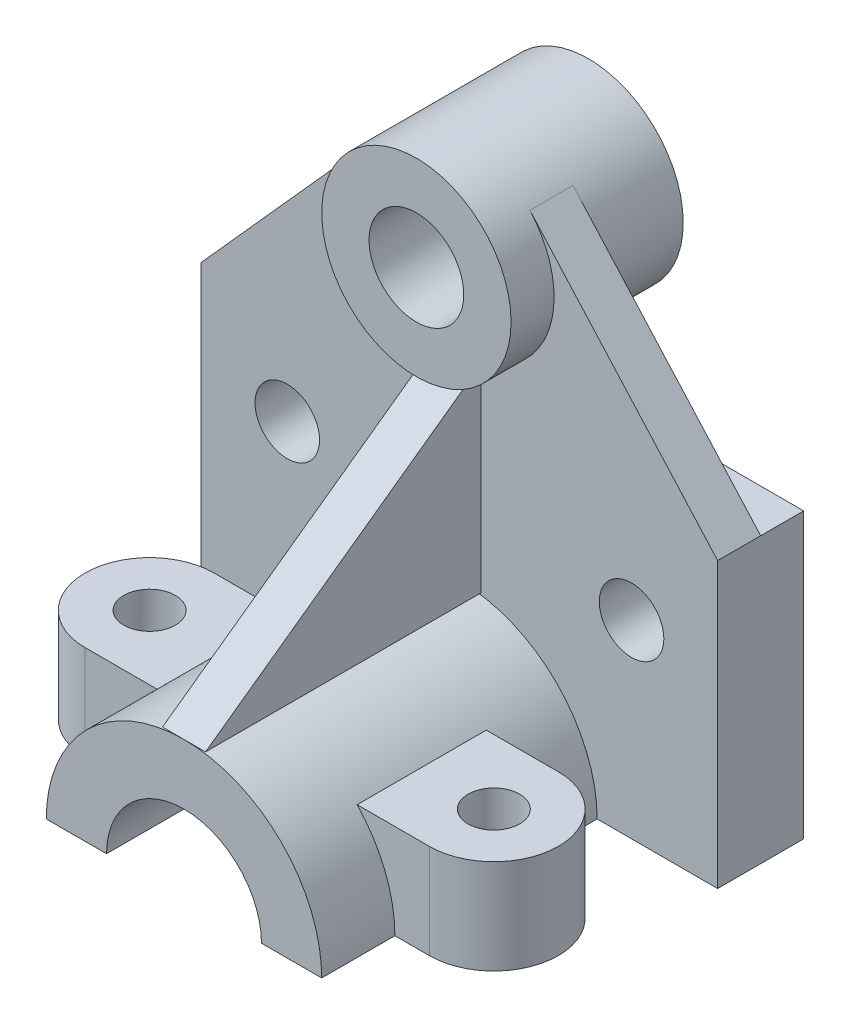
ISO-10303-21;
HEADER;
FILE_DESCRIPTION(('STEP AP214'),'2;1');
FILE_NAME('part.step','',(''),(''),'','','');
FILE_SCHEMA(('AUTOMOTIVE_DESIGN { 1 0 10303 214 1 1 1 1 }'));
ENDSEC;
DATA;
#1=APPLICATION_CONTEXT('core data for automotive mechanical design processes');
#2=APPLICATION_PROTOCOL_DEFINITION('international standard','automotive_design',2000,#1);
#3=PRODUCT_CONTEXT('',#1,'mechanical');
#4=PRODUCT('Part','Part','',(#3));
#5=PRODUCT_RELATED_PRODUCT_CATEGORY('part','',(#4));
#6=PRODUCT_DEFINITION_FORMATION('','',#4);
#7=PRODUCT_DEFINITION_CONTEXT('part definition',#1,'design');
#8=PRODUCT_DEFINITION('design','',#6,#7);
#9=PRODUCT_DEFINITION_SHAPE('','',#8);
#10=(LENGTH_UNIT() NAMED_UNIT(*) SI_UNIT(.MILLI.,.METRE.));
#11=(NAMED_UNIT(*) PLANE_ANGLE_UNIT() SI_UNIT($,.RADIAN.));
#12=(NAMED_UNIT(*) SI_UNIT($,.STERADIAN.) SOLID_ANGLE_UNIT());
#13=UNCERTAINTY_MEASURE_WITH_UNIT(LENGTH_MEASURE(1.E-05),#10,'distance_accuracy_value','');
#14=(GEOMETRIC_REPRESENTATION_CONTEXT(3) GLOBAL_UNCERTAINTY_ASSIGNED_CONTEXT((#13)) GLOBAL_UNIT_ASSIGNED_CONTEXT((#10,
#11,#12)) REPRESENTATION_CONTEXT('',''));
#15=CARTESIAN_POINT('',(0.,0.,0.));
#16=DIRECTION('',(0.,0.,1.));
#17=DIRECTION('',(1.,0.,0.));
#18=AXIS2_PLACEMENT_3D('',#15,#16,#17);
#19=CARTESIAN_POINT('',(120.,32.,0.));
#20=DIRECTION('',(0.,0.,-1.));
#21=DIRECTION('',(-1.,0.,0.));
#22=AXIS2_PLACEMENT_3D('',#19,#20,#21);
#23=PLANE('',#22);
#24=DIRECTION('',(0.,1.,0.));
#25=VECTOR('',#24,1.);
#26=CARTESIAN_POINT('',(65.,32.,0.));
#27=LINE('',#26,#25);
#28=CARTESIAN_POINT('',(65.,32.,0.));
#29=VERTEX_POINT('',#28);
#30=CARTESIAN_POINT('',(65.,78.,0.));
#31=VERTEX_POINT('',#30);
#32=EDGE_CURVE('E89',#29,#31,#27,.T.);
#33=ORIENTED_EDGE('',*,*,#32,.F.);
#34=DIRECTION('',(-1.,0.,0.));
#35=VECTOR('',#34,1.);
#36=CARTESIAN_POINT('',(120.,32.,0.));
#37=LINE('',#36,#35);
#38=CARTESIAN_POINT('',(55.,32.,0.));
#39=VERTEX_POINT('',#38);
#40=EDGE_CURVE('E58',#29,#39,#37,.T.);
#41=ORIENTED_EDGE('',*,*,#40,.T.);
#42=DIRECTION('',(0.,-1.,0.));
#43=VECTOR('',#42,1.);
#44=CARTESIAN_POINT('',(55.,32.,0.));
#45=LINE('',#44,#43);
#46=CARTESIAN_POINT('',(55.,78.,0.));
#47=VERTEX_POINT('',#46);
#48=EDGE_CURVE('E101',#47,#39,#45,.T.);
#49=ORIENTED_EDGE('',*,*,#48,.F.);
#50=DIRECTION('',(-1.,0.,0.));
#51=VECTOR('',#50,1.);
#52=CARTESIAN_POINT('',(120.,78.,0.));
#53=LINE('',#52,#51);
#54=EDGE_CURVE('E12',#31,#47,#53,.T.);
#55=ORIENTED_EDGE('',*,*,#54,.F.);
#56=EDGE_LOOP('',(#33,#41,#49,#55));
#57=FACE_BOUND('',#56,.T.);
#58=ADVANCED_FACE('F60',(#57),#23,.T.);
#59=CARTESIAN_POINT('',(120.,78.,0.));
#60=DIRECTION('',(0.,0.812015371342713,0.583636048152576));
#61=DIRECTION('',(0.,-0.583636048152576,0.812015371342713));
#62=AXIS2_PLACEMENT_3D('',#59,#60,#61);
#63=PLANE('',#62);
#64=DIRECTION('',(0.,-0.583636048152575,0.812015371342713));
#65=VECTOR('',#64,1.);
#66=CARTESIAN_POINT('',(65.,78.,0.));
#67=LINE('',#66,#65);
#68=CARTESIAN_POINT('',(65.,32.,64.));
#69=VERTEX_POINT('',#68);
#70=EDGE_CURVE('E71',#31,#69,#67,.T.);
#71=ORIENTED_EDGE('',*,*,#70,.F.);
#72=ORIENTED_EDGE('',*,*,#54,.T.);
#73=DIRECTION('',(0.,0.583636048152575,-0.812015371342713));
#74=VECTOR('',#73,1.);
#75=CARTESIAN_POINT('',(55.,78.,0.));
#76=LINE('',#75,#74);
#77=CARTESIAN_POINT('',(55.,32.,64.));
#78=VERTEX_POINT('',#77);
#79=EDGE_CURVE('E110',#78,#47,#76,.T.);
#80=ORIENTED_EDGE('',*,*,#79,.F.);
#81=DIRECTION('',(-1.,0.,0.));
#82=VECTOR('',#81,1.);
#83=CARTESIAN_POINT('',(120.,32.,64.));
#84=LINE('',#83,#82);
#85=EDGE_CURVE('E61',#69,#78,#84,.T.);
#86=ORIENTED_EDGE('',*,*,#85,.F.);
#87=EDGE_LOOP('',(#71,#72,#80,#86));
#88=FACE_BOUND('',#87,.T.);
#89=ADVANCED_FACE('F100',(#88),#63,.T.);
#90=CARTESIAN_POINT('',(120.,32.,64.));
#91=DIRECTION('',(0.,-1.,0.));
#92=DIRECTION('',(0.,0.,-1.));
#93=AXIS2_PLACEMENT_3D('',#90,#91,#92);
#94=PLANE('',#93);
#95=DIRECTION('',(0.,0.,-1.));
#96=VECTOR('',#95,1.);
#97=CARTESIAN_POINT('',(65.,32.,64.));
#98=LINE('',#97,#96);
#99=EDGE_CURVE('E95',#69,#29,#98,.T.);
#100=ORIENTED_EDGE('',*,*,#99,.F.);
#101=ORIENTED_EDGE('',*,*,#85,.T.);
#102=DIRECTION('',(0.,0.,1.));
#103=VECTOR('',#102,1.);
#104=CARTESIAN_POINT('',(55.,32.,64.));
#105=LINE('',#104,#103);
#106=EDGE_CURVE('E104',#39,#78,#105,.T.);
#107=ORIENTED_EDGE('',*,*,#106,.F.);
#108=ORIENTED_EDGE('',*,*,#40,.F.);
#109=EDGE_LOOP('',(#100,#101,#107,#108));
#110=FACE_BOUND('',#109,.T.);
#111=ADVANCED_FACE('F115',(#110),#94,.T.);
#112=CARTESIAN_POINT('',(55.,0.,0.));
#113=DIRECTION('',(-1.,0.,0.));
#114=DIRECTION('',(0.,0.,1.));
#115=AXIS2_PLACEMENT_3D('',#112,#113,#114);
#116=PLANE('',#115);
#117=ORIENTED_EDGE('',*,*,#48,.T.);
#118=ORIENTED_EDGE('',*,*,#106,.T.);
#119=ORIENTED_EDGE('',*,*,#79,.T.);
#120=EDGE_LOOP('',(#117,#118,#119));
#121=FACE_BOUND('',#120,.T.);
#122=ADVANCED_FACE('F114',(#121),#116,.T.);
#123=CARTESIAN_POINT('',(65.,0.,0.));
#124=DIRECTION('',(-1.,0.,0.));
#125=DIRECTION('',(0.,0.,1.));
#126=AXIS2_PLACEMENT_3D('',#123,#124,#125);
#127=PLANE('',#126);
#128=ORIENTED_EDGE('',*,*,#32,.T.);
#129=ORIENTED_EDGE('',*,*,#70,.T.);
#130=ORIENTED_EDGE('',*,*,#99,.T.);
#131=EDGE_LOOP('',(#128,#129,#130));
#132=FACE_BOUND('',#131,.T.);
#133=ADVANCED_FACE('F93',(#132),#127,.F.);
#134=CLOSED_SHELL('',(#58,#89,#111,#122,#133));
#135=MANIFOLD_SOLID_BREP('B2',#134);
#136=CARTESIAN_POINT('',(60.,0.,64.));
#137=DIRECTION('',(0.,0.,-1.));
#138=DIRECTION('',(-1.,0.,0.));
#139=AXIS2_PLACEMENT_3D('',#136,#137,#138);
#140=CYLINDRICAL_SURFACE('',#139,32.);
#141=CARTESIAN_POINT('',(60.,0.,17.));
#142=DIRECTION('',(0.,0.,1.));
#143=DIRECTION('',(1.,0.,0.));
#144=AXIS2_PLACEMENT_3D('',#141,#142,#143);
#145=CIRCLE('',#144,32.);
#146=CARTESIAN_POINT('',(36.7620999227555,22.,17.));
#147=VERTEX_POINT('',#146);
#148=CARTESIAN_POINT('',(28.,0.,17.));
#149=VERTEX_POINT('',#148);
#150=EDGE_CURVE('E318',#147,#149,#145,.T.);
#151=ORIENTED_EDGE('',*,*,#150,.F.);
#152=DIRECTION('',(0.,0.,-1.));
#153=VECTOR('',#152,1.);
#154=CARTESIAN_POINT('',(36.7620999227555,22.,64.));
#155=LINE('',#154,#153);
#156=CARTESIAN_POINT('',(36.7620999227555,22.,47.));
#157=VERTEX_POINT('',#156);
#158=EDGE_CURVE('E54',#157,#147,#155,.T.);
#159=ORIENTED_EDGE('',*,*,#158,.F.);
#160=CARTESIAN_POINT('',(60.,0.,47.));
#161=DIRECTION('',(0.,0.,-1.));
#162=DIRECTION('',(-1.,0.,0.));
#163=AXIS2_PLACEMENT_3D('',#160,#161,#162);
#164=CIRCLE('',#163,32.);
#165=CARTESIAN_POINT('',(28.,0.,47.));
#166=VERTEX_POINT('',#165);
#167=EDGE_CURVE('E296',#166,#157,#164,.T.);
#168=ORIENTED_EDGE('',*,*,#167,.F.);
#169=DIRECTION('',(0.,0.,-1.));
#170=VECTOR('',#169,1.);
#171=CARTESIAN_POINT('',(28.,0.,64.));
#172=LINE('',#171,#170);
#173=CARTESIAN_POINT('',(28.,0.,64.));
#174=VERTEX_POINT('',#173);
#175=EDGE_CURVE('E409',#174,#166,#172,.T.);
#176=ORIENTED_EDGE('',*,*,#175,.F.);
#177=CARTESIAN_POINT('',(60.,0.,64.));
#178=DIRECTION('',(0.,0.,1.));
#179=DIRECTION('',(1.,0.,0.));
#180=AXIS2_PLACEMENT_3D('',#177,#178,#179);
#181=CIRCLE('',#180,32.);
#182=CARTESIAN_POINT('',(92.,0.,64.));
#183=VERTEX_POINT('',#182);
#184=EDGE_CURVE('E396',#183,#174,#181,.T.);
#185=ORIENTED_EDGE('',*,*,#184,.F.);
#186=DIRECTION('',(0.,0.,-1.));
#187=VECTOR('',#186,1.);
#188=CARTESIAN_POINT('',(92.,0.,64.));
#189=LINE('',#188,#187);
#190=CARTESIAN_POINT('',(92.,0.,47.));
#191=VERTEX_POINT('',#190);
#192=EDGE_CURVE('E407',#183,#191,#189,.T.);
#193=ORIENTED_EDGE('',*,*,#192,.T.);
#194=CARTESIAN_POINT('',(60.,0.,47.));
#195=DIRECTION('',(0.,0.,1.));
#196=DIRECTION('',(1.,0.,0.));
#197=AXIS2_PLACEMENT_3D('',#194,#195,#196);
#198=CIRCLE('',#197,32.);
#199=CARTESIAN_POINT('',(83.2379000772445,22.,47.));
#200=VERTEX_POINT('',#199);
#201=EDGE_CURVE('E178',#191,#200,#198,.T.);
#202=ORIENTED_EDGE('',*,*,#201,.T.);
#203=DIRECTION('',(0.,0.,-1.));
#204=VECTOR('',#203,1.);
#205=CARTESIAN_POINT('',(83.2379000772445,22.,64.));
#206=LINE('',#205,#204);
#207=CARTESIAN_POINT('',(83.2379000772445,22.,17.));
#208=VERTEX_POINT('',#207);
#209=EDGE_CURVE('E162',#208,#200,#206,.F.);
#210=ORIENTED_EDGE('',*,*,#209,.F.);
#211=CARTESIAN_POINT('',(60.,0.,17.));
#212=DIRECTION('',(0.,0.,-1.));
#213=DIRECTION('',(-1.,0.,0.));
#214=AXIS2_PLACEMENT_3D('',#211,#212,#213);
#215=CIRCLE('',#214,32.);
#216=CARTESIAN_POINT('',(92.,0.,17.));
#217=VERTEX_POINT('',#216);
#218=EDGE_CURVE('E345',#208,#217,#215,.T.);
#219=ORIENTED_EDGE('',*,*,#218,.T.);
#220=CARTESIAN_POINT('',(92.,0.,0.));
#221=VERTEX_POINT('',#220);
#222=EDGE_CURVE('E401',#217,#221,#189,.T.);
#223=ORIENTED_EDGE('',*,*,#222,.T.);
#224=CARTESIAN_POINT('',(60.,0.,0.));
#225=DIRECTION('',(0.,0.,1.));
#226=DIRECTION('',(1.,0.,0.));
#227=AXIS2_PLACEMENT_3D('',#224,#225,#226);
#228=CIRCLE('',#227,32.);
#229=CARTESIAN_POINT('',(28.,0.,0.));
#230=VERTEX_POINT('',#229);
#231=EDGE_CURVE('E394',#221,#230,#228,.T.);
#232=ORIENTED_EDGE('',*,*,#231,.T.);
#233=EDGE_CURVE('E408',#149,#230,#172,.T.);
#234=ORIENTED_EDGE('',*,*,#233,.F.);
#235=EDGE_LOOP('',(#151,#159,#168,#176,#185,#193,#202,#210,#219,#223,#232,#234));
#236=FACE_BOUND('',#235,.T.);
#237=ADVANCED_FACE('F154',(#236),#140,.T.);
#238=CARTESIAN_POINT('',(0.,66.,-20.));
#239=DIRECTION('',(-1.,0.,0.));
#240=DIRECTION('',(0.,0.,1.));
#241=AXIS2_PLACEMENT_3D('',#238,#239,#240);
#242=PLANE('',#241);
#243=DIRECTION('',(0.,-1.,0.));
#244=VECTOR('',#243,1.);
#245=CARTESIAN_POINT('',(0.,66.,0.));
#246=LINE('',#245,#244);
#247=CARTESIAN_POINT('',(0.,66.,0.));
#248=VERTEX_POINT('',#247);
#249=CARTESIAN_POINT('',(0.,0.,0.));
#250=VERTEX_POINT('',#249);
#251=EDGE_CURVE('E415',#248,#250,#246,.T.);
#252=ORIENTED_EDGE('',*,*,#251,.F.);
#253=DIRECTION('',(0.,0.,1.));
#254=VECTOR('',#253,1.);
#255=CARTESIAN_POINT('',(0.,66.,-10.));
#256=LINE('',#255,#254);
#257=CARTESIAN_POINT('',(0.,66.,-10.));
#258=VERTEX_POINT('',#257);
#259=EDGE_CURVE('E378',#258,#248,#256,.T.);
#260=ORIENTED_EDGE('',*,*,#259,.F.);
#261=DIRECTION('',(0.,0.,1.));
#262=VECTOR('',#261,1.);
#263=CARTESIAN_POINT('',(0.,66.,-20.));
#264=LINE('',#263,#262);
#265=CARTESIAN_POINT('',(0.,66.,-20.));
#266=VERTEX_POINT('',#265);
#267=EDGE_CURVE('E434',#266,#258,#264,.T.);
#268=ORIENTED_EDGE('',*,*,#267,.F.);
#269=DIRECTION('',(0.,-1.,0.));
#270=VECTOR('',#269,1.);
#271=CARTESIAN_POINT('',(0.,66.,-20.));
#272=LINE('',#271,#270);
#273=CARTESIAN_POINT('',(0.,0.,-20.));
#274=VERTEX_POINT('',#273);
#275=EDGE_CURVE('E413',#266,#274,#272,.T.);
#276=ORIENTED_EDGE('',*,*,#275,.T.);
#277=DIRECTION('',(0.,0.,1.));
#278=VECTOR('',#277,1.);
#279=CARTESIAN_POINT('',(0.,0.,-20.));
#280=LINE('',#279,#278);
#281=EDGE_CURVE('E426',#274,#250,#280,.T.);
#282=ORIENTED_EDGE('',*,*,#281,.T.);
#283=EDGE_LOOP('',(#252,#260,#268,#276,#282));
#284=FACE_BOUND('',#283,.T.);
#285=ADVANCED_FACE('F160',(#284),#242,.T.);
#286=CARTESIAN_POINT('',(120.,66.,-20.));
#287=DIRECTION('',(0.,1.,0.));
#288=DIRECTION('',(0.,0.,1.));
#289=AXIS2_PLACEMENT_3D('',#286,#287,#288);
#290=PLANE('',#289);
#291=DIRECTION('',(-1.,0.,0.));
#292=VECTOR('',#291,1.);
#293=CARTESIAN_POINT('',(0.,66.,-10.));
#294=LINE('',#293,#292);
#295=CARTESIAN_POINT('',(120.,66.,-10.));
#296=VERTEX_POINT('',#295);
#297=EDGE_CURVE('E362',#296,#258,#294,.T.);
#298=ORIENTED_EDGE('',*,*,#297,.F.);
#299=DIRECTION('',(0.,0.,1.));
#300=VECTOR('',#299,1.);
#301=CARTESIAN_POINT('',(120.,66.,-20.));
#302=LINE('',#301,#300);
#303=CARTESIAN_POINT('',(120.,66.,-20.));
#304=VERTEX_POINT('',#303);
#305=EDGE_CURVE('E437',#304,#296,#302,.T.);
#306=ORIENTED_EDGE('',*,*,#305,.F.);
#307=DIRECTION('',(-1.,0.,0.));
#308=VECTOR('',#307,1.);
#309=CARTESIAN_POINT('',(120.,66.,-20.));
#310=LINE('',#309,#308);
#311=EDGE_CURVE('E421',#304,#266,#310,.T.);
#312=ORIENTED_EDGE('',*,*,#311,.T.);
#313=ORIENTED_EDGE('',*,*,#267,.T.);
#314=EDGE_LOOP('',(#298,#306,#312,#313));
#315=FACE_BOUND('',#314,.T.);
#316=ADVANCED_FACE('F500',(#315),#290,.T.);
#317=CARTESIAN_POINT('',(120.,0.,-20.));
#318=DIRECTION('',(1.,0.,0.));
#319=DIRECTION('',(0.,0.,-1.));
#320=AXIS2_PLACEMENT_3D('',#317,#318,#319);
#321=PLANE('',#320);
#322=DIRECTION('',(0.,1.,0.));
#323=VECTOR('',#322,1.);
#324=CARTESIAN_POINT('',(120.,0.,0.));
#325=LINE('',#324,#323);
#326=CARTESIAN_POINT('',(120.,0.,0.));
#327=VERTEX_POINT('',#326);
#328=CARTESIAN_POINT('',(120.,66.,0.));
#329=VERTEX_POINT('',#328);
#330=EDGE_CURVE('E417',#327,#329,#325,.T.);
#331=ORIENTED_EDGE('',*,*,#330,.F.);
#332=DIRECTION('',(0.,0.,1.));
#333=VECTOR('',#332,1.);
#334=CARTESIAN_POINT('',(120.,0.,-20.));
#335=LINE('',#334,#333);
#336=CARTESIAN_POINT('',(120.,0.,-20.));
#337=VERTEX_POINT('',#336);
#338=EDGE_CURVE('E442',#337,#327,#335,.T.);
#339=ORIENTED_EDGE('',*,*,#338,.F.);
#340=DIRECTION('',(0.,1.,0.));
#341=VECTOR('',#340,1.);
#342=CARTESIAN_POINT('',(120.,0.,-20.));
#343=LINE('',#342,#341);
#344=EDGE_CURVE('E419',#337,#304,#343,.T.);
#345=ORIENTED_EDGE('',*,*,#344,.T.);
#346=ORIENTED_EDGE('',*,*,#305,.T.);
#347=DIRECTION('',(0.,0.,1.));
#348=VECTOR('',#347,1.);
#349=CARTESIAN_POINT('',(120.,66.,-10.));
#350=LINE('',#349,#348);
#351=EDGE_CURVE('E376',#296,#329,#350,.T.);
#352=ORIENTED_EDGE('',*,*,#351,.T.);
#353=EDGE_LOOP('',(#331,#339,#345,#346,#352));
#354=FACE_BOUND('',#353,.T.);
#355=ADVANCED_FACE('F478',(#354),#321,.T.);
#356=CARTESIAN_POINT('',(0.,0.,-20.));
#357=DIRECTION('',(0.,-1.,0.));
#358=DIRECTION('',(0.,0.,-1.));
#359=AXIS2_PLACEMENT_3D('',#356,#357,#358);
#360=PLANE('',#359);
#361=CARTESIAN_POINT('',(20.,0.,32.));
#362=DIRECTION('',(0.,-1.,0.));
#363=DIRECTION('',(0.,0.,-1.));
#364=AXIS2_PLACEMENT_3D('',#361,#362,#363);
#365=CIRCLE('',#364,6.);
#366=CARTESIAN_POINT('',(20.,0.,26.));
#367=VERTEX_POINT('',#366);
#368=EDGE_CURVE('E518',#367,#367,#365,.T.);
#369=ORIENTED_EDGE('',*,*,#368,.F.);
#370=EDGE_LOOP('',(#369));
#371=FACE_BOUND('',#370,.T.);
#372=CARTESIAN_POINT('',(100.,0.,32.));
#373=DIRECTION('',(0.,-1.,0.));
#374=DIRECTION('',(0.,0.,-1.));
#375=AXIS2_PLACEMENT_3D('',#372,#373,#374);
#376=CIRCLE('',#375,6.);
#377=CARTESIAN_POINT('',(100.,0.,26.));
#378=VERTEX_POINT('',#377);
#379=EDGE_CURVE('E511',#378,#378,#376,.T.);
#380=ORIENTED_EDGE('',*,*,#379,.F.);
#381=EDGE_LOOP('',(#380));
#382=FACE_BOUND('',#381,.T.);
#383=DIRECTION('',(-1.,0.,0.));
#384=VECTOR('',#383,1.);
#385=CARTESIAN_POINT('',(0.,0.,17.));
#386=LINE('',#385,#384);
#387=CARTESIAN_POINT('',(20.,0.,17.));
#388=VERTEX_POINT('',#387);
#389=EDGE_CURVE('E168',#149,#388,#386,.T.);
#390=ORIENTED_EDGE('',*,*,#389,.F.);
#391=ORIENTED_EDGE('',*,*,#233,.T.);
#392=DIRECTION('',(1.,0.,0.));
#393=VECTOR('',#392,1.);
#394=CARTESIAN_POINT('',(0.,0.,0.));
#395=LINE('',#394,#393);
#396=EDGE_CURVE('E429',#250,#230,#395,.T.);
#397=ORIENTED_EDGE('',*,*,#396,.F.);
#398=ORIENTED_EDGE('',*,*,#281,.F.);
#399=DIRECTION('',(1.,0.,0.));
#400=VECTOR('',#399,1.);
#401=CARTESIAN_POINT('',(0.,0.,-20.));
#402=LINE('',#401,#400);
#403=EDGE_CURVE('E418',#274,#337,#402,.T.);
#404=ORIENTED_EDGE('',*,*,#403,.T.);
#405=ORIENTED_EDGE('',*,*,#338,.T.);
#406=EDGE_CURVE('E427',#221,#327,#395,.T.);
#407=ORIENTED_EDGE('',*,*,#406,.F.);
#408=ORIENTED_EDGE('',*,*,#222,.F.);
#409=DIRECTION('',(1.,0.,0.));
#410=VECTOR('',#409,1.);
#411=CARTESIAN_POINT('',(0.,0.,17.));
#412=LINE('',#411,#410);
#413=CARTESIAN_POINT('',(100.,0.,17.));
#414=VERTEX_POINT('',#413);
#415=EDGE_CURVE('E319',#217,#414,#412,.T.);
#416=ORIENTED_EDGE('',*,*,#415,.T.);
#417=CARTESIAN_POINT('',(100.,0.,32.));
#418=DIRECTION('',(0.,-1.,0.));
#419=DIRECTION('',(0.,0.,-1.));
#420=AXIS2_PLACEMENT_3D('',#417,#418,#419);
#421=CIRCLE('',#420,15.);
#422=CARTESIAN_POINT('',(100.,0.,47.));
#423=VERTEX_POINT('',#422);
#424=EDGE_CURVE('E335',#414,#423,#421,.T.);
#425=ORIENTED_EDGE('',*,*,#424,.T.);
#426=DIRECTION('',(-1.,0.,0.));
#427=VECTOR('',#426,1.);
#428=CARTESIAN_POINT('',(0.,0.,47.));
#429=LINE('',#428,#427);
#430=EDGE_CURVE('E322',#423,#191,#429,.T.);
#431=ORIENTED_EDGE('',*,*,#430,.T.);
#432=ORIENTED_EDGE('',*,*,#192,.F.);
#433=DIRECTION('',(1.,0.,0.));
#434=VECTOR('',#433,1.);
#435=CARTESIAN_POINT('',(28.,0.,64.));
#436=LINE('',#435,#434);
#437=CARTESIAN_POINT('',(78.,0.,64.));
#438=VERTEX_POINT('',#437);
#439=EDGE_CURVE('E397',#438,#183,#436,.T.);
#440=ORIENTED_EDGE('',*,*,#439,.F.);
#441=DIRECTION('',(0.,0.,1.));
#442=VECTOR('',#441,1.);
#443=CARTESIAN_POINT('',(78.,0.,0.));
#444=LINE('',#443,#442);
#445=CARTESIAN_POINT('',(78.,0.,0.));
#446=VERTEX_POINT('',#445);
#447=EDGE_CURVE('E395',#446,#438,#444,.T.);
#448=ORIENTED_EDGE('',*,*,#447,.F.);
#449=DIRECTION('',(1.,0.,0.));
#450=VECTOR('',#449,1.);
#451=CARTESIAN_POINT('',(42.,0.,0.));
#452=LINE('',#451,#450);
#453=CARTESIAN_POINT('',(42.,0.,0.));
#454=VERTEX_POINT('',#453);
#455=EDGE_CURVE('E387',#454,#446,#452,.T.);
#456=ORIENTED_EDGE('',*,*,#455,.F.);
#457=DIRECTION('',(0.,0.,1.));
#458=VECTOR('',#457,1.);
#459=CARTESIAN_POINT('',(42.,0.,0.));
#460=LINE('',#459,#458);
#461=CARTESIAN_POINT('',(42.,0.,64.));
#462=VERTEX_POINT('',#461);
#463=EDGE_CURVE('E386',#454,#462,#460,.T.);
#464=ORIENTED_EDGE('',*,*,#463,.T.);
#465=EDGE_CURVE('E399',#174,#462,#436,.T.);
#466=ORIENTED_EDGE('',*,*,#465,.F.);
#467=ORIENTED_EDGE('',*,*,#175,.T.);
#468=DIRECTION('',(1.,0.,0.));
#469=VECTOR('',#468,1.);
#470=CARTESIAN_POINT('',(0.,0.,47.));
#471=LINE('',#470,#469);
#472=CARTESIAN_POINT('',(20.,0.,47.));
#473=VERTEX_POINT('',#472);
#474=EDGE_CURVE('E315',#473,#166,#471,.T.);
#475=ORIENTED_EDGE('',*,*,#474,.F.);
#476=CARTESIAN_POINT('',(20.,0.,32.));
#477=DIRECTION('',(0.,-1.,0.));
#478=DIRECTION('',(0.,0.,-1.));
#479=AXIS2_PLACEMENT_3D('',#476,#477,#478);
#480=CIRCLE('',#479,15.);
#481=EDGE_CURVE('E292',#473,#388,#480,.T.);
#482=ORIENTED_EDGE('',*,*,#481,.T.);
#483=EDGE_LOOP('',(#390,#391,#397,#398,#404,#405,#407,#408,#416,#425,#431,#432,#440,#448,#456,
#464,#466,#467,#475,#482));
#484=FACE_BOUND('',#483,.T.);
#485=ADVANCED_FACE('F473',(#371,#382,#484),#360,.T.);
#486=CARTESIAN_POINT('',(0.,0.,-20.));
#487=DIRECTION('',(0.,0.,1.));
#488=DIRECTION('',(1.,0.,0.));
#489=AXIS2_PLACEMENT_3D('',#486,#487,#488);
#490=PLANE('',#489);
#491=CARTESIAN_POINT('',(20.,44.,-20.));
#492=DIRECTION('',(0.,0.,1.));
#493=DIRECTION('',(1.,0.,0.));
#494=AXIS2_PLACEMENT_3D('',#491,#492,#493);
#495=CIRCLE('',#494,7.5);
#496=CARTESIAN_POINT('',(27.5,44.,-20.));
#497=VERTEX_POINT('',#496);
#498=EDGE_CURVE('E311',#497,#497,#495,.T.);
#499=ORIENTED_EDGE('',*,*,#498,.T.);
#500=EDGE_LOOP('',(#499));
#501=FACE_BOUND('',#500,.T.);
#502=CARTESIAN_POINT('',(100.,44.,-20.));
#503=DIRECTION('',(0.,0.,1.));
#504=DIRECTION('',(1.,0.,0.));
#505=AXIS2_PLACEMENT_3D('',#502,#503,#504);
#506=CIRCLE('',#505,7.5);
#507=CARTESIAN_POINT('',(107.5,44.,-20.));
#508=VERTEX_POINT('',#507);
#509=EDGE_CURVE('E506',#508,#508,#506,.T.);
#510=ORIENTED_EDGE('',*,*,#509,.T.);
#511=EDGE_LOOP('',(#510));
#512=FACE_BOUND('',#511,.T.);
#513=ORIENTED_EDGE('',*,*,#275,.F.);
#514=ORIENTED_EDGE('',*,*,#311,.F.);
#515=ORIENTED_EDGE('',*,*,#344,.F.);
#516=ORIENTED_EDGE('',*,*,#403,.F.);
#517=EDGE_LOOP('',(#513,#514,#515,#516));
#518=FACE_BOUND('',#517,.T.);
#519=ADVANCED_FACE('F498',(#501,#512,#518),#490,.F.);
#520=CARTESIAN_POINT('',(0.,0.,0.));
#521=DIRECTION('',(0.,0.,1.));
#522=DIRECTION('',(1.,0.,0.));
#523=AXIS2_PLACEMENT_3D('',#520,#521,#522);
#524=PLANE('',#523);
#525=CARTESIAN_POINT('',(20.,44.,0.));
#526=DIRECTION('',(0.,0.,1.));
#527=DIRECTION('',(1.,0.,0.));
#528=AXIS2_PLACEMENT_3D('',#525,#526,#527);
#529=CIRCLE('',#528,7.5);
#530=CARTESIAN_POINT('',(27.5,44.,0.));
#531=VERTEX_POINT('',#530);
#532=EDGE_CURVE('E507',#531,#531,#529,.T.);
#533=ORIENTED_EDGE('',*,*,#532,.F.);
#534=EDGE_LOOP('',(#533));
#535=FACE_BOUND('',#534,.T.);
#536=CARTESIAN_POINT('',(100.,44.,0.));
#537=DIRECTION('',(0.,0.,1.));
#538=DIRECTION('',(1.,0.,0.));
#539=AXIS2_PLACEMENT_3D('',#536,#537,#538);
#540=CIRCLE('',#539,7.5);
#541=CARTESIAN_POINT('',(107.5,44.,0.));
#542=VERTEX_POINT('',#541);
#543=EDGE_CURVE('E509',#542,#542,#540,.T.);
#544=ORIENTED_EDGE('',*,*,#543,.F.);
#545=EDGE_LOOP('',(#544));
#546=FACE_BOUND('',#545,.T.);
#547=DIRECTION('',(-0.667290225653567,0.744797794537021,0.));
#548=VECTOR('',#547,1.);
#549=CARTESIAN_POINT('',(99.368605602936,89.0277867926307,0.));
#550=LINE('',#549,#548);
#551=CARTESIAN_POINT('',(76.3855514798145,114.680384964378,0.));
#552=VERTEX_POINT('',#551);
#553=EDGE_CURVE('E361',#329,#552,#550,.T.);
#554=ORIENTED_EDGE('',*,*,#553,.T.);
#555=CARTESIAN_POINT('',(60.,100.,0.));
#556=DIRECTION('',(0.,0.,1.));
#557=DIRECTION('',(1.,0.,0.));
#558=AXIS2_PLACEMENT_3D('',#555,#556,#557);
#559=CIRCLE('',#558,22.);
#560=CARTESIAN_POINT('',(43.6144485201855,114.680384964378,0.));
#561=VERTEX_POINT('',#560);
#562=EDGE_CURVE('E355',#561,#552,#559,.T.);
#563=ORIENTED_EDGE('',*,*,#562,.F.);
#564=DIRECTION('',(0.667290225653567,0.744797794537022,0.));
#565=VECTOR('',#564,1.);
#566=CARTESIAN_POINT('',(-32.8017550332706,29.388232186684,0.));
#567=LINE('',#566,#565);
#568=EDGE_CURVE('E356',#248,#561,#567,.T.);
#569=ORIENTED_EDGE('',*,*,#568,.F.);
#570=ORIENTED_EDGE('',*,*,#251,.T.);
#571=ORIENTED_EDGE('',*,*,#396,.T.);
#572=ORIENTED_EDGE('',*,*,#231,.F.);
#573=ORIENTED_EDGE('',*,*,#406,.T.);
#574=ORIENTED_EDGE('',*,*,#330,.T.);
#575=EDGE_LOOP('',(#554,#563,#569,#570,#571,#572,#573,#574));
#576=FACE_BOUND('',#575,.T.);
#577=ADVANCED_FACE('F467',(#535,#546,#576),#524,.T.);
#578=CARTESIAN_POINT('',(60.,0.,64.));
#579=DIRECTION('',(0.,0.,1.));
#580=DIRECTION('',(1.,0.,0.));
#581=AXIS2_PLACEMENT_3D('',#578,#579,#580);
#582=PLANE('',#581);
#583=CARTESIAN_POINT('',(60.,0.,64.));
#584=DIRECTION('',(0.,0.,1.));
#585=DIRECTION('',(1.,0.,0.));
#586=AXIS2_PLACEMENT_3D('',#583,#584,#585);
#587=CIRCLE('',#586,18.);
#588=EDGE_CURVE('E374',#438,#462,#587,.T.);
#589=ORIENTED_EDGE('',*,*,#588,.F.);
#590=ORIENTED_EDGE('',*,*,#439,.T.);
#591=ORIENTED_EDGE('',*,*,#184,.T.);
#592=ORIENTED_EDGE('',*,*,#465,.T.);
#593=EDGE_LOOP('',(#589,#590,#591,#592));
#594=FACE_BOUND('',#593,.T.);
#595=ADVANCED_FACE('F548',(#594),#582,.T.);
#596=CARTESIAN_POINT('',(60.,0.,0.));
#597=DIRECTION('',(0.,0.,1.));
#598=DIRECTION('',(1.,0.,0.));
#599=AXIS2_PLACEMENT_3D('',#596,#597,#598);
#600=CYLINDRICAL_SURFACE('',#599,18.);
#601=ORIENTED_EDGE('',*,*,#588,.T.);
#602=ORIENTED_EDGE('',*,*,#463,.F.);
#603=CARTESIAN_POINT('',(60.,0.,0.));
#604=DIRECTION('',(0.,0.,1.));
#605=DIRECTION('',(1.,0.,0.));
#606=AXIS2_PLACEMENT_3D('',#603,#604,#605);
#607=CIRCLE('',#606,18.);
#608=EDGE_CURVE('E382',#446,#454,#607,.T.);
#609=ORIENTED_EDGE('',*,*,#608,.F.);
#610=ORIENTED_EDGE('',*,*,#447,.T.);
#611=EDGE_LOOP('',(#601,#602,#609,#610));
#612=FACE_BOUND('',#611,.T.);
#613=ADVANCED_FACE('F604',(#612),#600,.F.);
#614=CARTESIAN_POINT('',(60.,0.,0.));
#615=DIRECTION('',(0.,0.,1.));
#616=DIRECTION('',(1.,0.,0.));
#617=AXIS2_PLACEMENT_3D('',#614,#615,#616);
#618=PLANE('',#617);
#619=ORIENTED_EDGE('',*,*,#608,.T.);
#620=ORIENTED_EDGE('',*,*,#455,.T.);
#621=EDGE_LOOP('',(#619,#620));
#622=FACE_BOUND('',#621,.T.);
#623=ADVANCED_FACE('F602',(#622),#618,.T.);
#624=CARTESIAN_POINT('',(60.,100.,-10.));
#625=DIRECTION('',(0.,0.,1.));
#626=DIRECTION('',(1.,0.,0.));
#627=AXIS2_PLACEMENT_3D('',#624,#625,#626);
#628=CYLINDRICAL_SURFACE('',#627,22.);
#629=DIRECTION('',(0.,0.,1.));
#630=VECTOR('',#629,1.);
#631=CARTESIAN_POINT('',(43.6144485201855,114.680384964379,-10.));
#632=LINE('',#631,#630);
#633=CARTESIAN_POINT('',(43.6144485201855,114.680384964378,-10.));
#634=VERTEX_POINT('',#633);
#635=EDGE_CURVE('E369',#634,#561,#632,.T.);
#636=ORIENTED_EDGE('',*,*,#635,.T.);
#637=ORIENTED_EDGE('',*,*,#562,.T.);
#638=DIRECTION('',(0.,0.,1.));
#639=VECTOR('',#638,1.);
#640=CARTESIAN_POINT('',(76.3855514798145,114.680384964378,-10.));
#641=LINE('',#640,#639);
#642=CARTESIAN_POINT('',(76.3855514798145,114.680384964378,-10.));
#643=VERTEX_POINT('',#642);
#644=EDGE_CURVE('E373',#643,#552,#641,.T.);
#645=ORIENTED_EDGE('',*,*,#644,.F.);
#646=CARTESIAN_POINT('',(60.,100.,-10.));
#647=DIRECTION('',(0.,0.,1.));
#648=DIRECTION('',(1.,0.,0.));
#649=AXIS2_PLACEMENT_3D('',#646,#647,#648);
#650=CIRCLE('',#649,22.);
#651=EDGE_CURVE('E440',#643,#634,#650,.F.);
#652=ORIENTED_EDGE('',*,*,#651,.T.);
#653=EDGE_LOOP('',(#636,#637,#645,#652));
#654=FACE_BOUND('',#653,.T.);
#655=CARTESIAN_POINT('',(60.,100.,10.));
#656=DIRECTION('',(0.,0.,1.));
#657=DIRECTION('',(1.,0.,0.));
#658=AXIS2_PLACEMENT_3D('',#655,#656,#657);
#659=CIRCLE('',#658,22.);
#660=CARTESIAN_POINT('',(82.,100.,10.));
#661=VERTEX_POINT('',#660);
#662=EDGE_CURVE('E353',#661,#661,#659,.T.);
#663=ORIENTED_EDGE('',*,*,#662,.F.);
#664=EDGE_LOOP('',(#663));
#665=FACE_BOUND('',#664,.T.);
#666=CARTESIAN_POINT('',(60.,100.,-30.));
#667=DIRECTION('',(0.,0.,-1.));
#668=DIRECTION('',(-1.,0.,0.));
#669=AXIS2_PLACEMENT_3D('',#666,#667,#668);
#670=CIRCLE('',#669,22.);
#671=CARTESIAN_POINT('',(38.,100.,-30.));
#672=VERTEX_POINT('',#671);
#673=EDGE_CURVE('E349',#672,#672,#670,.T.);
#674=ORIENTED_EDGE('',*,*,#673,.F.);
#675=EDGE_LOOP('',(#674));
#676=FACE_BOUND('',#675,.T.);
#677=ADVANCED_FACE('F484',(#654,#665,#676),#628,.T.);
#678=CARTESIAN_POINT('',(99.368605602936,89.0277867926307,-10.));
#679=DIRECTION('',(0.744797794537021,0.667290225653567,0.));
#680=DIRECTION('',(-0.667290225653567,0.744797794537021,0.));
#681=AXIS2_PLACEMENT_3D('',#678,#679,#680);
#682=PLANE('',#681);
#683=ORIENTED_EDGE('',*,*,#553,.F.);
#684=ORIENTED_EDGE('',*,*,#351,.F.);
#685=DIRECTION('',(-0.667290225653567,0.744797794537021,0.));
#686=VECTOR('',#685,1.);
#687=CARTESIAN_POINT('',(99.368605602936,89.0277867926307,-10.));
#688=LINE('',#687,#686);
#689=EDGE_CURVE('E368',#296,#643,#688,.T.);
#690=ORIENTED_EDGE('',*,*,#689,.T.);
#691=ORIENTED_EDGE('',*,*,#644,.T.);
#692=EDGE_LOOP('',(#683,#684,#690,#691));
#693=FACE_BOUND('',#692,.T.);
#694=ADVANCED_FACE('F481',(#693),#682,.T.);
#695=CARTESIAN_POINT('',(-32.8017550332706,29.388232186684,-10.));
#696=DIRECTION('',(0.744797794537022,-0.667290225653567,0.));
#697=DIRECTION('',(0.667290225653567,0.744797794537022,0.));
#698=AXIS2_PLACEMENT_3D('',#695,#696,#697);
#699=PLANE('',#698);
#700=ORIENTED_EDGE('',*,*,#568,.T.);
#701=ORIENTED_EDGE('',*,*,#635,.F.);
#702=DIRECTION('',(0.667290225653567,0.744797794537022,0.));
#703=VECTOR('',#702,1.);
#704=CARTESIAN_POINT('',(-32.8017550332706,29.388232186684,-10.));
#705=LINE('',#704,#703);
#706=EDGE_CURVE('E357',#258,#634,#705,.T.);
#707=ORIENTED_EDGE('',*,*,#706,.F.);
#708=ORIENTED_EDGE('',*,*,#259,.T.);
#709=EDGE_LOOP('',(#700,#701,#707,#708));
#710=FACE_BOUND('',#709,.T.);
#711=ADVANCED_FACE('F487',(#710),#699,.F.);
#712=CARTESIAN_POINT('',(0.,0.,-10.));
#713=DIRECTION('',(0.,0.,1.));
#714=DIRECTION('',(1.,0.,0.));
#715=AXIS2_PLACEMENT_3D('',#712,#713,#714);
#716=PLANE('',#715);
#717=ORIENTED_EDGE('',*,*,#651,.F.);
#718=ORIENTED_EDGE('',*,*,#689,.F.);
#719=ORIENTED_EDGE('',*,*,#297,.T.);
#720=ORIENTED_EDGE('',*,*,#706,.T.);
#721=EDGE_LOOP('',(#717,#718,#719,#720));
#722=FACE_BOUND('',#721,.T.);
#723=ADVANCED_FACE('F494',(#722),#716,.F.);
#724=CARTESIAN_POINT('',(60.,100.,10.));
#725=DIRECTION('',(0.,0.,1.));
#726=DIRECTION('',(1.,0.,0.));
#727=AXIS2_PLACEMENT_3D('',#724,#725,#726);
#728=PLANE('',#727);
#729=CARTESIAN_POINT('',(60.,100.,10.));
#730=DIRECTION('',(0.,0.,1.));
#731=DIRECTION('',(1.,0.,0.));
#732=AXIS2_PLACEMENT_3D('',#729,#730,#731);
#733=CIRCLE('',#732,11.);
#734=CARTESIAN_POINT('',(71.,100.,10.));
#735=VERTEX_POINT('',#734);
#736=EDGE_CURVE('E344',#735,#735,#733,.T.);
#737=ORIENTED_EDGE('',*,*,#736,.F.);
#738=EDGE_LOOP('',(#737));
#739=FACE_BOUND('',#738,.T.);
#740=ORIENTED_EDGE('',*,*,#662,.T.);
#741=EDGE_LOOP('',(#740));
#742=FACE_BOUND('',#741,.T.);
#743=ADVANCED_FACE('F591',(#739,#742),#728,.T.);
#744=CARTESIAN_POINT('',(60.,100.,-30.));
#745=DIRECTION('',(0.,0.,-1.));
#746=DIRECTION('',(-1.,0.,0.));
#747=AXIS2_PLACEMENT_3D('',#744,#745,#746);
#748=PLANE('',#747);
#749=CARTESIAN_POINT('',(60.,100.,-30.));
#750=DIRECTION('',(0.,0.,-1.));
#751=DIRECTION('',(-1.,0.,0.));
#752=AXIS2_PLACEMENT_3D('',#749,#750,#751);
#753=CIRCLE('',#752,11.);
#754=CARTESIAN_POINT('',(49.,100.,-30.));
#755=VERTEX_POINT('',#754);
#756=EDGE_CURVE('E346',#755,#755,#753,.T.);
#757=ORIENTED_EDGE('',*,*,#756,.F.);
#758=EDGE_LOOP('',(#757));
#759=FACE_BOUND('',#758,.T.);
#760=ORIENTED_EDGE('',*,*,#673,.T.);
#761=EDGE_LOOP('',(#760));
#762=FACE_BOUND('',#761,.T.);
#763=ADVANCED_FACE('F582',(#759,#762),#748,.T.);
#764=CARTESIAN_POINT('',(60.,100.,-40.));
#765=DIRECTION('',(0.,0.,1.));
#766=DIRECTION('',(1.,0.,0.));
#767=AXIS2_PLACEMENT_3D('',#764,#765,#766);
#768=CYLINDRICAL_SURFACE('',#767,11.);
#769=ORIENTED_EDGE('',*,*,#756,.T.);
#770=EDGE_LOOP('',(#769));
#771=FACE_BOUND('',#770,.T.);
#772=ORIENTED_EDGE('',*,*,#736,.T.);
#773=EDGE_LOOP('',(#772));
#774=FACE_BOUND('',#773,.T.);
#775=ADVANCED_FACE('F571',(#771,#774),#768,.F.);
#776=CARTESIAN_POINT('',(0.,22.,0.));
#777=DIRECTION('',(0.,-1.,0.));
#778=DIRECTION('',(0.,0.,-1.));
#779=AXIS2_PLACEMENT_3D('',#776,#777,#778);
#780=PLANE('',#779);
#781=CARTESIAN_POINT('',(100.,22.,32.));
#782=DIRECTION('',(0.,1.,0.));
#783=DIRECTION('',(0.,0.,1.));
#784=AXIS2_PLACEMENT_3D('',#781,#782,#783);
#785=CIRCLE('',#784,6.);
#786=CARTESIAN_POINT('',(100.,22.,38.));
#787=VERTEX_POINT('',#786);
#788=EDGE_CURVE('E525',#787,#787,#785,.T.);
#789=ORIENTED_EDGE('',*,*,#788,.F.);
#790=EDGE_LOOP('',(#789));
#791=FACE_BOUND('',#790,.T.);
#792=DIRECTION('',(1.,0.,0.));
#793=VECTOR('',#792,1.);
#794=CARTESIAN_POINT('',(0.,22.,17.));
#795=LINE('',#794,#793);
#796=CARTESIAN_POINT('',(100.,22.,17.));
#797=VERTEX_POINT('',#796);
#798=EDGE_CURVE('E321',#208,#797,#795,.T.);
#799=ORIENTED_EDGE('',*,*,#798,.F.);
#800=ORIENTED_EDGE('',*,*,#209,.T.);
#801=DIRECTION('',(-1.,0.,0.));
#802=VECTOR('',#801,1.);
#803=CARTESIAN_POINT('',(0.,22.,47.));
#804=LINE('',#803,#802);
#805=CARTESIAN_POINT('',(100.,22.,47.));
#806=VERTEX_POINT('',#805);
#807=EDGE_CURVE('E330',#806,#200,#804,.T.);
#808=ORIENTED_EDGE('',*,*,#807,.F.);
#809=CARTESIAN_POINT('',(100.,22.,32.));
#810=DIRECTION('',(0.,-1.,0.));
#811=DIRECTION('',(0.,0.,-1.));
#812=AXIS2_PLACEMENT_3D('',#809,#810,#811);
#813=CIRCLE('',#812,15.);
#814=EDGE_CURVE('E323',#797,#806,#813,.T.);
#815=ORIENTED_EDGE('',*,*,#814,.F.);
#816=EDGE_LOOP('',(#799,#800,#808,#815));
#817=FACE_BOUND('',#816,.T.);
#818=ADVANCED_FACE('F451',(#791,#817),#780,.F.);
#819=CARTESIAN_POINT('',(0.,22.,17.));
#820=DIRECTION('',(0.,0.,-1.));
#821=DIRECTION('',(-1.,0.,0.));
#822=AXIS2_PLACEMENT_3D('',#819,#820,#821);
#823=PLANE('',#822);
#824=ORIENTED_EDGE('',*,*,#218,.F.);
#825=ORIENTED_EDGE('',*,*,#798,.T.);
#826=DIRECTION('',(0.,-1.,0.));
#827=VECTOR('',#826,1.);
#828=CARTESIAN_POINT('',(100.,22.,17.));
#829=LINE('',#828,#827);
#830=EDGE_CURVE('E329',#797,#414,#829,.T.);
#831=ORIENTED_EDGE('',*,*,#830,.T.);
#832=ORIENTED_EDGE('',*,*,#415,.F.);
#833=EDGE_LOOP('',(#824,#825,#831,#832));
#834=FACE_BOUND('',#833,.T.);
#835=ADVANCED_FACE('F463',(#834),#823,.T.);
#836=CARTESIAN_POINT('',(0.,22.,47.));
#837=DIRECTION('',(0.,0.,1.));
#838=DIRECTION('',(1.,0.,0.));
#839=AXIS2_PLACEMENT_3D('',#836,#837,#838);
#840=PLANE('',#839);
#841=ORIENTED_EDGE('',*,*,#201,.F.);
#842=ORIENTED_EDGE('',*,*,#430,.F.);
#843=DIRECTION('',(0.,-1.,0.));
#844=VECTOR('',#843,1.);
#845=CARTESIAN_POINT('',(100.,22.,47.));
#846=LINE('',#845,#844);
#847=EDGE_CURVE('E340',#806,#423,#846,.T.);
#848=ORIENTED_EDGE('',*,*,#847,.F.);
#849=ORIENTED_EDGE('',*,*,#807,.T.);
#850=EDGE_LOOP('',(#841,#842,#848,#849));
#851=FACE_BOUND('',#850,.T.);
#852=ADVANCED_FACE('F454',(#851),#840,.T.);
#853=CARTESIAN_POINT('',(100.,22.,32.));
#854=DIRECTION('',(0.,-1.,0.));
#855=DIRECTION('',(0.,0.,-1.));
#856=AXIS2_PLACEMENT_3D('',#853,#854,#855);
#857=CYLINDRICAL_SURFACE('',#856,15.);
#858=ORIENTED_EDGE('',*,*,#424,.F.);
#859=ORIENTED_EDGE('',*,*,#830,.F.);
#860=ORIENTED_EDGE('',*,*,#814,.T.);
#861=ORIENTED_EDGE('',*,*,#847,.T.);
#862=EDGE_LOOP('',(#858,#859,#860,#861));
#863=FACE_BOUND('',#862,.T.);
#864=ADVANCED_FACE('F459',(#863),#857,.T.);
#865=CARTESIAN_POINT('',(0.,22.,0.));
#866=DIRECTION('',(0.,-1.,0.));
#867=DIRECTION('',(0.,0.,-1.));
#868=AXIS2_PLACEMENT_3D('',#865,#866,#867);
#869=PLANE('',#868);
#870=CARTESIAN_POINT('',(20.,22.,32.));
#871=DIRECTION('',(0.,1.,0.));
#872=DIRECTION('',(0.,0.,1.));
#873=AXIS2_PLACEMENT_3D('',#870,#871,#872);
#874=CIRCLE('',#873,6.);
#875=CARTESIAN_POINT('',(20.,22.,38.));
#876=VERTEX_POINT('',#875);
#877=EDGE_CURVE('E521',#876,#876,#874,.T.);
#878=ORIENTED_EDGE('',*,*,#877,.F.);
#879=EDGE_LOOP('',(#878));
#880=FACE_BOUND('',#879,.T.);
#881=DIRECTION('',(1.,0.,0.));
#882=VECTOR('',#881,1.);
#883=CARTESIAN_POINT('',(0.,22.,47.));
#884=LINE('',#883,#882);
#885=CARTESIAN_POINT('',(20.,22.,47.));
#886=VERTEX_POINT('',#885);
#887=EDGE_CURVE('E300',#886,#157,#884,.T.);
#888=ORIENTED_EDGE('',*,*,#887,.T.);
#889=ORIENTED_EDGE('',*,*,#158,.T.);
#890=DIRECTION('',(-1.,0.,0.));
#891=VECTOR('',#890,1.);
#892=CARTESIAN_POINT('',(0.,22.,17.));
#893=LINE('',#892,#891);
#894=CARTESIAN_POINT('',(20.,22.,17.));
#895=VERTEX_POINT('',#894);
#896=EDGE_CURVE('E303',#147,#895,#893,.T.);
#897=ORIENTED_EDGE('',*,*,#896,.T.);
#898=CARTESIAN_POINT('',(20.,22.,32.));
#899=DIRECTION('',(0.,-1.,0.));
#900=DIRECTION('',(0.,0.,-1.));
#901=AXIS2_PLACEMENT_3D('',#898,#899,#900);
#902=CIRCLE('',#901,15.);
#903=EDGE_CURVE('E289',#886,#895,#902,.T.);
#904=ORIENTED_EDGE('',*,*,#903,.F.);
#905=EDGE_LOOP('',(#888,#889,#897,#904));
#906=FACE_BOUND('',#905,.T.);
#907=ADVANCED_FACE('F304',(#880,#906),#869,.F.);
#908=CARTESIAN_POINT('',(0.,22.,17.));
#909=DIRECTION('',(0.,0.,1.));
#910=DIRECTION('',(1.,0.,0.));
#911=AXIS2_PLACEMENT_3D('',#908,#909,#910);
#912=PLANE('',#911);
#913=ORIENTED_EDGE('',*,*,#896,.F.);
#914=ORIENTED_EDGE('',*,*,#150,.T.);
#915=ORIENTED_EDGE('',*,*,#389,.T.);
#916=DIRECTION('',(0.,-1.,0.));
#917=VECTOR('',#916,1.);
#918=CARTESIAN_POINT('',(20.,22.,17.));
#919=LINE('',#918,#917);
#920=EDGE_CURVE('E294',#895,#388,#919,.T.);
#921=ORIENTED_EDGE('',*,*,#920,.F.);
#922=EDGE_LOOP('',(#913,#914,#915,#921));
#923=FACE_BOUND('',#922,.T.);
#924=ADVANCED_FACE('F505',(#923),#912,.F.);
#925=CARTESIAN_POINT('',(0.,22.,47.));
#926=DIRECTION('',(0.,0.,-1.));
#927=DIRECTION('',(-1.,0.,0.));
#928=AXIS2_PLACEMENT_3D('',#925,#926,#927);
#929=PLANE('',#928);
#930=ORIENTED_EDGE('',*,*,#474,.T.);
#931=ORIENTED_EDGE('',*,*,#167,.T.);
#932=ORIENTED_EDGE('',*,*,#887,.F.);
#933=DIRECTION('',(0.,-1.,0.));
#934=VECTOR('',#933,1.);
#935=CARTESIAN_POINT('',(20.,22.,47.));
#936=LINE('',#935,#934);
#937=EDGE_CURVE('E281',#886,#473,#936,.T.);
#938=ORIENTED_EDGE('',*,*,#937,.T.);
#939=EDGE_LOOP('',(#930,#931,#932,#938));
#940=FACE_BOUND('',#939,.T.);
#941=ADVANCED_FACE('F298',(#940),#929,.F.);
#942=CARTESIAN_POINT('',(20.,22.,32.));
#943=DIRECTION('',(0.,-1.,0.));
#944=DIRECTION('',(0.,0.,-1.));
#945=AXIS2_PLACEMENT_3D('',#942,#943,#944);
#946=CYLINDRICAL_SURFACE('',#945,15.);
#947=ORIENTED_EDGE('',*,*,#481,.F.);
#948=ORIENTED_EDGE('',*,*,#937,.F.);
#949=ORIENTED_EDGE('',*,*,#903,.T.);
#950=ORIENTED_EDGE('',*,*,#920,.T.);
#951=EDGE_LOOP('',(#947,#948,#949,#950));
#952=FACE_BOUND('',#951,.T.);
#953=ADVANCED_FACE('F290',(#952),#946,.T.);
#954=CARTESIAN_POINT('',(100.,44.,-30.));
#955=DIRECTION('',(0.,0.,1.));
#956=DIRECTION('',(1.,0.,0.));
#957=AXIS2_PLACEMENT_3D('',#954,#955,#956);
#958=CYLINDRICAL_SURFACE('',#957,7.5);
#959=ORIENTED_EDGE('',*,*,#543,.T.);
#960=EDGE_LOOP('',(#959));
#961=FACE_BOUND('',#960,.T.);
#962=ORIENTED_EDGE('',*,*,#509,.F.);
#963=EDGE_LOOP('',(#962));
#964=FACE_BOUND('',#963,.T.);
#965=ADVANCED_FACE('F810',(#961,#964),#958,.F.);
#966=CARTESIAN_POINT('',(20.,44.,-30.));
#967=DIRECTION('',(0.,0.,1.));
#968=DIRECTION('',(1.,0.,0.));
#969=AXIS2_PLACEMENT_3D('',#966,#967,#968);
#970=CYLINDRICAL_SURFACE('',#969,7.5);
#971=ORIENTED_EDGE('',*,*,#532,.T.);
#972=EDGE_LOOP('',(#971));
#973=FACE_BOUND('',#972,.T.);
#974=ORIENTED_EDGE('',*,*,#498,.F.);
#975=EDGE_LOOP('',(#974));
#976=FACE_BOUND('',#975,.T.);
#977=ADVANCED_FACE('F820',(#973,#976),#970,.F.);
#978=CARTESIAN_POINT('',(20.,-33.,32.));
#979=DIRECTION('',(0.,1.,0.));
#980=DIRECTION('',(0.,0.,1.));
#981=AXIS2_PLACEMENT_3D('',#978,#979,#980);
#982=CYLINDRICAL_SURFACE('',#981,6.);
#983=ORIENTED_EDGE('',*,*,#368,.T.);
#984=EDGE_LOOP('',(#983));
#985=FACE_BOUND('',#984,.T.);
#986=ORIENTED_EDGE('',*,*,#877,.T.);
#987=EDGE_LOOP('',(#986));
#988=FACE_BOUND('',#987,.T.);
#989=ADVANCED_FACE('F526',(#985,#988),#982,.F.);
#990=CARTESIAN_POINT('',(100.,-33.,32.));
#991=DIRECTION('',(0.,1.,0.));
#992=DIRECTION('',(0.,0.,1.));
#993=AXIS2_PLACEMENT_3D('',#990,#991,#992);
#994=CYLINDRICAL_SURFACE('',#993,6.);
#995=ORIENTED_EDGE('',*,*,#379,.T.);
#996=EDGE_LOOP('',(#995));
#997=FACE_BOUND('',#996,.T.);
#998=ORIENTED_EDGE('',*,*,#788,.T.);
#999=EDGE_LOOP('',(#998));
#1000=FACE_BOUND('',#999,.T.);
#1001=ADVANCED_FACE('F566',(#997,#1000),#994,.F.);
#1002=CLOSED_SHELL('',(#237,#285,#316,#355,#485,#519,#577,#595,#613,#623,#677,#694,#711,#723,
#743,#763,#775,#818,#835,#852,#864,#907,#924,#941,#953,#965,#977,#989,#1001));
#1003=MANIFOLD_SOLID_BREP('B6',#1002);
#1004=ADVANCED_BREP_SHAPE_REPRESENTATION('',(#18,#135,#1003),#14);
#1005=SHAPE_DEFINITION_REPRESENTATION(#9,#1004);
ENDSEC;
END-ISO-10303-21;
